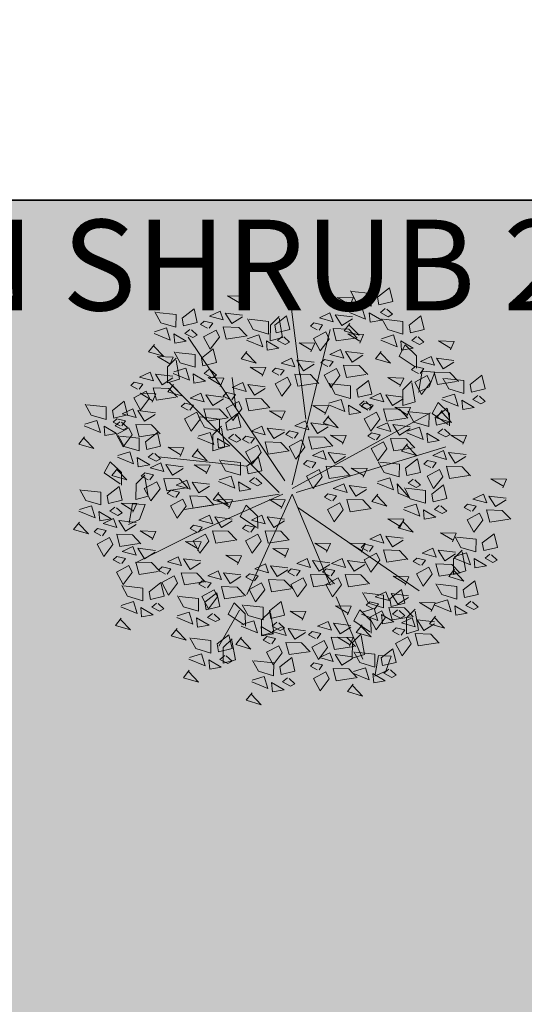
# Model space of a CAD drawing. Units: inches. Extents: x 1704 to 6393, y -157 to 1172.
# Tile 73 of 122: x 1954 to 1987, y 980 to 1045. Entities that reach past the tile are written whole.
import ezdxf

# ---------------------------------------------------------------- set-up
doc = ezdxf.new("R2010")
doc.units = ezdxf.units.IN
doc.header["$MEASUREMENT"] = 0
for name, color, linetype, lineweight in [('A-ANNO-DIMS', 7, 'Continuous', 13), ('C-PROP', 7, 'Continuous', 35), ('L-shrub', 74, 'Continuous', 18)]:
    doc.layers.add(name, color=color, linetype=linetype, lineweight=lineweight)
doc.layers.add('L-HRDS-PATT', color=9, linetype='Continuous', lineweight=13, true_color=0xc5c1ba)
doc.styles.get("Standard").update_dxf_attribs({"font": 'arial.ttf'})
doc.dimstyles.get("Standard").update_dxf_attribs({"dimtxt": 6, "dimasz": 2, "dimexe": 0.18, "dimexo": 0.0625, "dimgap": 0.09, "dimtad": 0, "dimtih": 1, "dimtoh": 1, "dimdec": 1, "dimzin": 0, "dimdsep": 46, "dimlunit": 3, "dimtxsty": 'Standard', "dimblk": 'ARCHTICK', "dimcen": 0.09, "dimadec": 0, "dimazin": 0, "dimtfac": 1, "dimtdec": 1, "dimtofl": 0, "dimtmove": 0, "dimatfit": 3, "dimfxl": 1, "dimtolj": 1, "dimtzin": 0, "dimarcsym": 0})

# ---------------------------------------------------------------- blocks, each defined once
blk = doc.blocks.new('flower shrub 3')
at = {"layer": 'L-shrub'}
for p, q in [((-123.5, 236), (-109, 242.8)), ((-130.4, 216.9), (-123.5, 236)), ((-109.8, 240.6), (-114, 215.7)), ((-114, 215.7), (-130.4, 216.9)), ((-96, 214.8), (-80.2, 219.2)), ((-80.2, 219.2), (-80.3, 198.9)), ((71.1, 221.6), (86.9, 226)), ((75.6, 196.7), (71.1, 221.6)), ((86.9, 226), (86.9, 205.7)), ((-91.6, 189.9), (-96, 214.8)), ((86.9, 205.7), (75.5, 194.4)), ((-80.3, 198.9), (-91.6, 187.7)), ((-166.1, 183.2), (-150.2, 187.7)), ((-161.6, 158.3), (-166.1, 183.2)), ((-150.2, 187.7), (-150.3, 167.3)), ((-104.3, 171), (-104.5, 187)), ((-102.9, 185.4), (-82, 171.2)), ((21.4, 185.5), (37.3, 189.9)), ((25.9, 160.6), (21.4, 185.5)), ((37.3, 189.9), (37.2, 169.6)), ((-150.3, 167.3), (-161.6, 156.1)), ((-89.8, 156.8), (-104.3, 171)), ((-82, 171.2), (-89.8, 156.8)), ((37.2, 169.6), (25.8, 158.3)), ((58.3, 162), (58.1, 177.9)), ((59.8, 176.3), (80.7, 162.2)), ((72.8, 147.7), (58.3, 162)), ((80.7, 162.2), (72.8, 147.7)), ((-227, 106.5), (-211.2, 110.9)), ((-222.6, 81.6), (-227, 106.5)), ((-211.2, 110.9), (-211.3, 90.6)), ((-211.3, 90.6), (-222.6, 79.4)), ((42.5, 35.6), (42.3, 51.6)), ((43.9, 50), (64.8, 35.8)), ((188.1, 20.6), (195.1, 39.7)), ((195.1, 39.7), (209.5, 46.5)), ((208.7, 44.3), (204.5, 19.5)), ((57, 21.4), (42.5, 35.6)), ((64.8, 35.8), (57, 21.4)), ((184.1, 9.5), (199.9, 13.9)), ((204.5, 19.5), (188.1, 20.6)), ((199.9, 13.9), (199.8, -6.4)), ((188.5, -15.4), (184.1, 9.5)), ((199.8, -6.4), (188.5, -17.7)), ((218.7, -20.8), (218.5, -4.8)), ((220.1, -6.4), (241, -20.6)), ((233.2, -35), (218.7, -20.8)), ((241, -20.6), (233.2, -35)), ((84.7, -53.7), (100.5, -49.2)), ((100.5, -49.2), (100.4, -69.6)), ((89.1, -78.6), (84.7, -53.7)), ((100.4, -69.6), (89.1, -80.8)), ((-206, -97.5), (-206.1, -81.5)), ((-204.5, -83.1), (-183.6, -97.3)), ((-191.5, -111.7), (-206, -97.5)), ((-183.6, -97.3), (-191.5, -111.7)), ((-161.5, -112.4), (-145.7, -107.9)), ((-157.1, -137.2), (-161.5, -112.4)), ((-145.7, -107.9), (-145.8, -128.2)), ((-179.9, -131.8), (-165.5, -125)), ((-166.2, -127.1), (-170.5, -152)), ((-186.9, -150.9), (-179.9, -131.8)), ((-145.8, -128.2), (-157.1, -139.5)), ((143.4, -141.7), (159.2, -137.2)), ((159.2, -137.2), (159.2, -157.6)), ((-170.5, -152), (-186.9, -150.9)), ((147.8, -166.6), (143.4, -141.7)), ((-163.1, -171.9), (-163.2, -156)), ((-161.6, -157.6), (-140.7, -171.7)), ((159.2, -157.6), (147.8, -168.8)), ((-148.6, -186.2), (-163.1, -171.9)), ((-140.7, -171.7), (-148.6, -186.2)), ((10.1, -195.8), (26, -191.4)), ((14.6, -220.7), (10.1, -195.8)), ((26, -191.4), (25.9, -211.7)), ((25.9, -211.7), (14.5, -223))]:
    blk.add_line(p, q, dxfattribs=at)
for points in [[(-81.5, 253.1), (-74, 262.7), (-93.5, 268.4), (-80.9, 255.3)], [(49.5, 264.4), (57, 273.9), (37.6, 279.7), (50.2, 266.6)], [(-50.4, 246.2), (-38.7, 261.6), (-30.1, 245.6), (-46.1, 237), (-50.4, 246.2)], [(3.7, 245), (10, 250.2), (-0.2, 255.6), (-5.8, 252.5), (1.6, 245.7)], [(24.3, 250.7), (23.1, 262.8), (8.2, 260.2), (24.3, 250.7)], [(49.4, 248), (33.8, 243.2), (29, 258.7), (50, 250.1)], [(-127.3, 233.7), (-121, 238.9), (-131.2, 244.3), (-136.8, 241.3), (-129.5, 234.4)], [(-106.8, 239.4), (-107.9, 251.5), (-122.8, 248.9), (-106.8, 239.4)], [(-81.7, 236.7), (-97.2, 231.9), (-102, 247.4), (-81, 238.9)], [(-84.3, 244.8), (-59.4, 248.7), (-55.3, 232.7), (-75.6, 233.3), (-86.6, 244.9)], [(130.8, 235.1), (138.4, 244.6), (118.9, 250.4), (131.5, 237.2)], [(-84.4, 211.6), (-109.5, 214.3), (-109.3, 230.8), (-89.8, 225), (-82.2, 211)], [(-37.1, 234.5), (-41.8, 227.9), (-30.6, 225.3), (-26, 229.7), (-34.9, 234.5)], [(13.5, 230.4), (-1.8, 218.4), (-6, 236.1), (11.8, 240.3), (13.5, 230.4)], [(46.7, 222.9), (21.5, 225.6), (21.7, 242.1), (41.2, 236.3), (48.8, 222.3)], [(105.6, 221.4), (104.4, 233.5), (89.5, 230.8), (105.6, 221.4)], [(-117.5, 219.1), (-132.8, 207.1), (-137, 224.8), (-119.3, 229), (-117.5, 219.1)], [(-59.4, 140), (-93.7, 220.8)], [(-80.5, 219.9), (-66.7, 228.5), (-58, 214.8), (-80.5, 217.6)], [(-55.5, 223.7), (-51.3, 212.3), (-37.6, 218.7), (-55.5, 223.7)], [(-48.1, 205.5), (-36.4, 221), (-27.8, 205), (-43.9, 196.4), (-48.1, 205.5)], [(10.6, 212.3), (22.3, 227.8), (30.9, 211.8), (14.9, 203.2), (10.6, 212.3)], [(85, 215.7), (91.3, 220.9), (81.1, 226.3), (75.5, 223.2), (82.9, 216.3)], [(130.7, 218.7), (115.1, 213.8), (110.3, 229.4), (131.3, 220.8)], [(-156.6, 201), (-144.8, 216.5), (-136.2, 200.5), (-152.3, 191.9), (-156.6, 201)], [(-82.1, 204.2), (-57.1, 208), (-53, 192.1), (-73.3, 192.7), (-84.3, 204.3)], [(-76.4, 204), (-81.2, 192.8), (-60.9, 192.3), (-76.4, 201.7)], [(-23.3, 211), (1.6, 214.8), (5.7, 198.9), (-14.6, 199.5), (-25.6, 211)], [(63.1, 192.2), (70.6, 201.7), (51.1, 207.5), (63.7, 194.4)], [(94.8, 201), (79.5, 189.1), (75.4, 206.8), (93.1, 211), (94.8, 201)], [(128, 193.6), (102.9, 196.3), (103, 212.7), (122.5, 207), (130.1, 192.9)], [(-190.5, 199.7), (-165.5, 203.5), (-161.4, 187.6), (-181.8, 188.2), (-192.7, 199.8)], [(-92.8, 176.4), (-85.3, 186), (-104.8, 191.7), (-92.2, 178.6)], [(-34.9, 193.9), (-39.6, 187.3), (-28.3, 184.7), (-23.7, 189.1), (-32.6, 193.8)], [(-19.5, 186), (-5.7, 194.7), (3, 180.9), (-19.5, 183.8)], [(23.9, 200.7), (19.2, 194), (30.4, 191.5), (35, 195.9), (26.1, 200.6)], [(65.7, 157.2), (92.6, 203.7)], [(146.6, 180.9), (154.2, 190.5), (134.7, 196.2), (147.3, 183.1)], [(-187.7, 165.1), (-180.1, 174.7), (-199.6, 180.4), (-187, 167.3)], [(-186.6, 174.8), (-172.8, 183.4), (-164.2, 169.6), (-186.7, 172.5)], [(-161.7, 178.6), (-157.5, 167.2), (-143.7, 173.6), (-161.7, 178.6)], [(-143.3, 189.4), (-148, 182.7), (-136.8, 180.2), (-132.1, 184.6), (-141, 189.3)], [(-122.7, 167.2), (-111, 182.7), (-102.3, 166.6), (-118.4, 158), (-122.7, 167.2)], [(-78.2, 179.3), (-64.4, 187.9), (-55.7, 174.2), (-78.3, 177)], [(-53.2, 183.1), (-49, 171.7), (-35.3, 178.1), (-53.2, 183.1)], [(5.5, 189.9), (9.7, 178.5), (23.4, 184.9), (5.5, 189.9)], [(17.3, 172.8), (23.5, 178), (13.3, 183.4), (7.7, 180.4), (15.1, 173.5)], [(37.8, 178.5), (36.7, 190.6), (21.8, 188), (37.8, 178.5)], [(62.9, 175.8), (47.4, 171), (42.5, 186.5), (63.6, 177.9)], [(121.4, 167.2), (120.3, 179.3), (105.3, 176.7), (121.4, 167.2)], [(218.9, 167.4), (226.5, 176.9), (207, 182.7), (219.6, 169.6)], [(-156.6, 165.8), (-131.6, 169.7), (-127.5, 153.8), (-147.9, 154.3), (-158.9, 165.9)], [(-138.6, 157), (-132.3, 162.2), (-142.5, 167.6), (-148.1, 164.6), (-140.8, 157.7)], [(-118.1, 162.7), (-119.2, 174.8), (-134.1, 172.2), (-118.1, 162.7)], [(-92.9, 160), (-108.5, 155.2), (-113.3, 170.7), (-92.3, 162.2)], [(-15.4, 170.1), (-20.2, 159), (0.1, 158.4), (-15.4, 167.9)], [(27.1, 158.2), (11.8, 146.2), (7.6, 163.9), (25.3, 168.1), (27.1, 158.2)], [(60.2, 150.7), (35.1, 153.4), (35.3, 169.9), (54.7, 164.1), (62.4, 150.1)], [(100.9, 161.5), (107.1, 166.7), (96.9, 172.1), (91.3, 169.1), (98.7, 162.2)], [(146.5, 164.5), (130.9, 159.7), (126.1, 175.2), (147.1, 166.7)], [(193.7, 153.7), (192.5, 165.8), (177.6, 163.1), (193.7, 153.7)], [(-233.5, 145.7), (-227.2, 151), (-237.4, 156.3), (-243, 153.3), (-235.6, 146.4)], [(-212.9, 151.4), (-214.1, 163.5), (-229, 160.9), (-212.9, 151.4)], [(-187.8, 148.7), (-203.4, 143.9), (-208.2, 159.4), (-187.2, 150.9)], [(-182.5, 158.9), (-187.4, 147.7), (-167, 147.1), (-182.6, 156.6)], [(-95.7, 134.9), (-120.8, 137.6), (-120.6, 154.1), (-101.1, 148.3), (-93.5, 134.3)], [(-109.4, 155.5), (-114.1, 148.9), (-102.9, 146.3), (-98.3, 150.7), (-107.2, 155.5)], [(-74.1, 163.4), (-78.9, 152.2), (-58.6, 151.7), (-74.2, 161.1)], [(110.7, 146.9), (95.3, 134.9), (91.2, 152.6), (108.9, 156.8), (110.7, 146.9)], [(94.2, 140.1), (105.9, 155.6), (114.5, 139.6), (98.5, 131), (94.2, 140.1)], [(143.8, 139.4), (118.7, 142.1), (118.8, 158.6), (138.3, 152.8), (146, 138.8)], [(173.1, 148), (179.4, 153.2), (169.2, 158.6), (163.6, 155.5), (171, 148.6)], [(218.8, 151), (203.2, 146.2), (198.4, 161.7), (219.4, 153.1)], [(-223.7, 131.1), (-239, 119.1), (-243.2, 136.9), (-225.4, 141), (-223.7, 131.1)], [(-190.5, 123.6), (-215.6, 126.4), (-215.5, 142.8), (-196, 137), (-188.4, 123)], [(-152.8, 140.9), (-139, 149.6), (-130.3, 135.8), (-152.8, 138.7)], [(-128.8, 142.4), (-144.1, 130.4), (-148.3, 148.1), (-130.6, 152.3), (-128.8, 142.4)], [(-127.8, 144.8), (-123.6, 133.4), (-109.9, 139.8), (-127.8, 144.8)], [(33.2, 131.1), (44.9, 146.6), (53.5, 130.5), (37.5, 121.9), (33.2, 131.1)], [(60.3, 138.8), (85.2, 142.6), (89.3, 126.7), (69, 127.3), (58, 138.8)], [(182.9, 133.3), (167.6, 121.4), (163.4, 139.1), (181.2, 143.3), (182.9, 133.3)], [(216.1, 125.9), (191, 128.6), (191.1, 145), (210.6, 139.3), (218.2, 125.2)], [(-9.9, 24.3), (-166.8, 132)], [(-66.2, 124.3), (-54.5, 139.8), (-45.9, 123.8), (-61.9, 115.2), (-66.2, 124.3)], [(-21, 124.3), (-9.3, 139.8), (-0.7, 123.8), (-16.7, 115.2), (-21, 124.3)], [(-0.7, 129.8), (24.2, 133.6), (28.3, 117.7), (8, 118.2), (-3, 129.8)], [(-2.5, 7.1), (56.3, 136.9)], [(107.4, 128.5), (102.7, 121.8), (114, 119.3), (118.6, 123.7), (109.7, 128.4)], [(146.1, 122.1), (157.9, 137.6), (166.5, 121.5), (150.4, 112.9), (146.1, 122.1)], [(-212.5, 104.2), (-205, 113.8), (-224.5, 119.5), (-211.9, 106.4)], [(-183.7, 110.8), (-171.9, 126.3), (-163.3, 110.2), (-179.4, 101.6), (-183.7, 110.8)], [(-148.7, 125), (-153.5, 113.9), (-133.2, 113.3), (-148.7, 122.8)], [(-100.1, 123), (-75.2, 126.8), (-71.1, 110.9), (-91.4, 111.5), (-102.4, 123)], [(-54.9, 123), (-30, 126.8), (-25.9, 110.9), (-46.2, 111.5), (-57.2, 123)], [(-2.5, 7.1), (-51.6, 124.7)], [(46.4, 119.4), (41.7, 112.8), (53, 110.2), (57.6, 114.6), (48.7, 119.4)], [(64.1, 113.8), (77.9, 122.5), (86.6, 108.7), (64, 111.6)], [(89.1, 117.7), (93.3, 106.3), (107, 112.7), (89.1, 117.7)], [(112.2, 120.7), (137.2, 124.6), (141.3, 108.7), (120.9, 109.2), (110, 120.8)], [(204.9, 108.5), (216.6, 124), (225.2, 108), (209.2, 99.4), (204.9, 108.5)], [(-237.8, 90.5), (-238.9, 102.6), (-253.8, 100), (-237.8, 90.5)], [(-217.6, 109.4), (-192.6, 113.3), (-188.5, 97.4), (-208.9, 97.9), (-219.9, 109.5)], [(-115.9, 92.7), (-104.2, 108.2), (-95.6, 92.2), (-111.6, 83.6), (-115.9, 92.7)], [(-96.3, 98.1), (-82.5, 106.7), (-73.8, 92.9), (-96.3, 95.8)], [(-53, 112.7), (-57.6, 106), (-46.4, 103.5), (-41.8, 107.9), (-50.7, 112.6)], [(-51.1, 98.1), (-37.3, 106.7), (-28.6, 92.9), (-51.2, 95.8)], [(-7.8, 112.7), (-12.5, 106), (-1.2, 103.5), (3.4, 107.9), (-5.5, 112.6)], [(3.1, 104.8), (16.9, 113.5), (25.6, 99.7), (3.1, 102.6)], [(28.1, 108.7), (32.3, 97.3), (46, 103.7), (28.1, 108.7)], [(116.1, 95.8), (129.9, 104.5), (138.5, 90.7), (116, 93.5)], [(159.4, 110.4), (154.7, 103.8), (165.9, 101.2), (170.6, 105.6), (161.6, 110.4)], [(170.9, 107.2), (195.9, 111), (200, 95.1), (179.7, 95.7), (168.7, 107.3)], [(-258.3, 84.8), (-252.1, 90), (-262.2, 95.4), (-267.9, 92.4), (-260.5, 85.5)], [(-212.7, 87.8), (-228.2, 83), (-233.1, 98.5), (-212, 90)], [(-213.7, 84.5), (-200, 93.2), (-191.3, 79.4), (-213.8, 82.3)], [(-170.4, 99.1), (-175.1, 92.5), (-163.9, 89.9), (-159.2, 94.3), (-168.2, 99.1)], [(-149.8, 91.4), (-124.9, 95.2), (-120.8, 79.3), (-141.1, 79.9), (-152.1, 91.5)], [(-71.3, 101.9), (-67.1, 90.5), (-53.4, 96.9), (-71.3, 101.9)], [(-26.1, 101.9), (-21.9, 90.5), (-8.2, 96.9), (-26.1, 101.9)], [(68.2, 97.9), (63.4, 86.8), (83.7, 86.2), (68.1, 95.7)], [(122.1, 56.8), (200.5, 95.9)], [(141, 99.6), (145.2, 88.2), (159, 94.6), (141, 99.6)], [(174.8, 82.3), (188.6, 90.9), (197.3, 77.1), (174.7, 80)], [(218.1, 96.9), (213.4, 90.2), (224.7, 87.7), (229.3, 92.1), (220.4, 96.8)], [(-248.5, 70.2), (-263.8, 58.2), (-268, 75.9), (-250.3, 80.1), (-248.5, 70.2)], [(-215.4, 62.7), (-240.5, 65.4), (-240.3, 81.9), (-220.8, 76.1), (-213.2, 62.1)], [(-188.8, 88.4), (-184.6, 77), (-170.8, 83.4), (-188.8, 88.4)], [(-102.6, 81.1), (-107.3, 74.5), (-96.1, 71.9), (-91.5, 76.3), (-100.4, 81)], [(-92.2, 82.1), (-97, 71), (-76.7, 70.4), (-92.3, 79.9)], [(-47, 82.1), (-51.8, 71), (-31.5, 70.4), (-47.1, 79.9)], [(7.2, 88.9), (2.4, 77.8), (22.7, 77.2), (7.1, 86.7)], [(37.7, 67.9), (49.4, 83.4), (58, 67.4), (42, 58.8), (37.7, 67.9)], [(105.5, 67.9), (117.2, 83.4), (125.8, 67.4), (109.8, 58.8), (105.5, 67.9)], [(120.2, 79.9), (115.3, 68.7), (135.7, 68.2), (120.1, 77.6)], [(199.8, 86.1), (204, 74.7), (217.7, 81.1), (199.8, 86.1)], [(229.7, 72.4), (241.4, 87.9), (250.1, 71.9), (234, 63.3), (229.7, 72.4)], [(-209.7, 68.6), (-214.5, 57.5), (-194.2, 56.9), (-209.7, 66.3)], [(-146, 66.5), (-132.2, 75.1), (-123.5, 61.3), (-146, 64.2)], [(-121, 70.3), (-116.8, 58.9), (-103.1, 65.3), (-121, 70.3)], [(3.8, 66.6), (28.7, 70.4), (32.8, 54.5), (12.5, 55.1), (1.5, 66.6)], [(71.6, 66.6), (96.5, 70.4), (100.6, 54.5), (80.3, 55.1), (69.3, 66.6)], [(178.9, 66.3), (174.1, 55.2), (194.4, 54.6), (178.8, 64.1)], [(195.8, 71.1), (220.8, 74.9), (224.8, 59), (204.5, 59.6), (193.5, 71.2)], [(-249.2, 40.8), (-237.5, 56.3), (-228.8, 40.3), (-244.9, 31.7), (-249.2, 40.8)], [(-147, 41), (-139.5, 50.6), (-159, 56.4), (-146.4, 43.2)], [(9.7, 7.1), (125, 58.6)], [(51, 56.3), (46.3, 49.6), (57.5, 47.1), (62.1, 51.5), (53.2, 56.2)], [(118.7, 56.3), (114, 49.6), (125.3, 47.1), (129.9, 51.5), (121, 56.2)], [(199.6, 46.2), (213.4, 54.8), (222.1, 41), (199.6, 43.9)], [(243, 60.8), (238.3, 54.1), (249.5, 51.6), (254.1, 56), (245.2, 60.7)], [(273.1, 43.3), (280.7, 52.8), (261.2, 58.6), (273.8, 45.5)], [(-283.1, 39.5), (-258.1, 43.3), (-254.1, 27.4), (-274.4, 28), (-285.4, 39.6)], [(-172.3, 27.3), (-173.4, 39.4), (-188.3, 36.8), (-172.3, 27.3)], [(-141.9, 50.6), (-146.7, 39.4), (-126.4, 38.9), (-141.9, 48.3)], [(-68.5, 27.3), (-56.7, 42.8), (-48.1, 26.8), (-64.2, 18.2), (-68.5, 27.3)], [(7.6, 41.6), (21.4, 50.3), (30.1, 36.5), (7.6, 39.4)], [(32.6, 45.5), (36.8, 34.1), (50.5, 40.5), (32.6, 45.5)], [(75.4, 41.6), (89.2, 50.3), (97.9, 36.5), (75.3, 39.4)], [(100.4, 45.5), (104.6, 34.1), (118.3, 40.5), (100.4, 45.5)], [(134.9, 22.8), (146.6, 38.3), (155.2, 22.2), (139.1, 13.7), (134.9, 22.8)], [(224.6, 50), (228.8, 38.6), (242.5, 45), (224.6, 50)], [(247.9, 29.6), (246.8, 41.7), (231.8, 39.1), (247.9, 29.6)], [(-235.9, 29.2), (-240.6, 22.6), (-229.4, 20), (-224.8, 24.4), (-233.7, 29.1)], [(-192.8, 21.7), (-186.5, 26.9), (-196.7, 32.2), (-202.4, 29.2), (-195, 22.3)], [(-147.2, 24.6), (-162.7, 19.8), (-167.5, 35.4), (-146.5, 26.8)], [(-102.4, 26), (-77.4, 29.8), (-73.3, 13.9), (-93.7, 14.4), (-104.6, 26)], [(11.7, 25.7), (6.9, 14.6), (27.2, 14), (11.7, 23.5)], [(14.6, 7.1), (137.2, 26.7)], [(79.5, 25.7), (74.7, 14.6), (95, 14), (79.4, 23.5)], [(203.7, 30.3), (198.9, 19.1), (219.2, 18.5), (203.7, 28)], [(227.4, 23.9), (233.6, 29.1), (223.4, 34.5), (217.8, 31.4), (225.2, 24.6)], [(273, 26.9), (257.4, 22.1), (252.6, 37.6), (273.6, 29)], [(-279.3, 14.6), (-265.5, 23.2), (-256.8, 9.5), (-279.3, 12.3)], [(-254.3, 18.4), (-250.1, 7), (-236.4, 13.4), (-254.3, 18.4)], [(-183, 7), (-198.3, -4.9), (-202.5, 12.8), (-184.8, 16.9), (-183, 7)], [(-149.9, -0.5), (-175, 2.3), (-174.8, 18.7), (-155.3, 12.9), (-147.7, -1.1)], [(-113.1, 7.2), (-105.6, 16.7), (-125.1, 22.5), (-112.5, 9.4)], [(-55.2, 15.7), (-59.9, 9), (-48.7, 6.5), (-44, 10.9), (-53, 15.6)], [(92.4, 4.9), (100, 14.5), (80.5, 20.3), (93.1, 7.1)], [(100.9, 21.5), (125.9, 25.3), (130, 9.4), (109.6, 9.9), (98.7, 21.5)], [(168.7, 0.2), (180.5, 15.7), (189.1, -0.3), (173, -8.9), (168.7, 0.2)], [(237.2, 9.2), (221.8, -2.7), (217.7, 15), (235.4, 19.2), (237.2, 9.2)], [(270.3, 1.8), (245.2, 4.5), (245.3, 20.9), (264.8, 15.2), (272.5, 1.2)], [(-7.4, 4.7), (-201.1, -54.1)], [(-138.4, -6.5), (-139.5, 5.6), (-154.3, 11.9), (-138.4, -6.5)], [(-113.3, -9.2), (-128.8, -14), (-133.7, 1.5), (-112.6, -7.1)], [(-98.5, 1), (-84.7, 9.7), (-76.1, -4.1), (-98.6, -1.2)], [(-73.6, 4.9), (-69.4, -6.5), (-55.6, -0.1), (-73.6, 4.9)], [(14.6, 4.7), (156.8, -137.4)], [(67.2, -8.8), (66, 3.3), (51.1, 0.7), (67.2, -8.8)], [(104.8, -3.5), (118.6, 5.2), (127.2, -8.6), (104.7, -5.7)], [(129.7, 0.4), (133.9, -11), (147.7, -4.6), (129.7, 0.4)], [(134.8, -1.1), (159.8, 2.7), (163.9, -13.2), (143.5, -12.6), (132.5, -1)], [(148.1, 11.2), (143.4, 4.5), (154.6, 2), (159.3, 6.3), (150.4, 11.1)], [(-275.2, -1.3), (-280, -12.5), (-259.7, -13), (-275.2, -3.6)], [(-197.2, -15.6), (-185.5, -0.1), (-176.9, -16.1), (-192.9, -24.7), (-197.2, -15.6)], [(-2.5, -0.2), (-181.5, -98.2)], [(-158.9, -12.2), (-152.7, -7), (-162.9, -1.6), (-168.5, -4.7), (-161.1, -11.5)], [(-2.5, -5.1), (-51.6, -205.9)], [(-41.3, -15.6), (-29.6, -0.1), (-21, -16.1), (-37.1, -24.7), (-41.3, -15.6)], [(7.3, -10), (132.3, -196.1)], [(46.6, -14.4), (52.9, -9.2), (42.7, -3.9), (37.1, -6.9), (44.5, -13.8)], [(92.3, -11.5), (76.7, -16.3), (71.9, -0.7), (92.9, -9.3)], [(182, -11.4), (177.3, -18.1), (188.5, -20.6), (193.1, -16.2), (184.2, -11.5)], [(223.5, -26.6), (231, -17.1), (211.5, -11.3), (224.1, -24.5)], [(-231.1, -16.9), (-206.2, -13.1), (-202.1, -29), (-222.4, -28.4), (-233.4, -16.8)], [(-149.1, -26.8), (-164.4, -38.8), (-168.6, -21.1), (-150.9, -16.9), (-149.1, -26.8)], [(-116, -34.3), (-141.1, -31.6), (-140.9, -15.2), (-121.5, -20.9), (-113.8, -34.9)], [(-94.4, -14.9), (-99.3, -26), (-78.9, -26.6), (-94.5, -17.1)], [(-75.3, -16.9), (-50.3, -13.1), (-46.2, -29), (-66.6, -28.4), (-77.5, -16.8)], [(56.4, -29.1), (41.1, -41), (36.9, -23.3), (54.7, -19.2), (56.4, -29.1)], [(89.6, -36.6), (64.5, -33.8), (64.6, -17.4), (84.1, -23.2), (91.7, -37.2)], [(108.9, -19.4), (104, -30.5), (124.4, -31.1), (108.8, -21.6)], [(138.6, -26), (152.4, -17.4), (161.1, -31.2), (138.6, -28.3)], [(163.6, -22.2), (167.8, -33.6), (181.6, -27.2), (163.6, -22.2)], [(-227.3, -41.8), (-213.5, -33.2), (-204.8, -46.9), (-227.4, -44.1)], [(-202.3, -38), (-198.1, -49.4), (-184.4, -43), (-202.3, -38)], [(-184, -27.2), (-188.7, -33.8), (-177.4, -36.4), (-172.8, -32), (-181.7, -27.3)], [(-124.9, -51.7), (-113.2, -36.2), (-104.6, -52.2), (-120.7, -60.8), (-124.9, -51.7)], [(-71.4, -41.8), (-57.6, -33.2), (-49, -46.9), (-71.5, -44.1)], [(-46.5, -38), (-42.3, -49.4), (-28.5, -43), (-46.5, -38)], [(-28.1, -27.2), (-32.8, -33.8), (-21.6, -36.4), (-16.9, -32), (-25.8, -27.3)], [(37.7, -47.1), (49.4, -31.7), (58, -47.7), (42, -56.3), (37.7, -47.1)], [(55.9, -29), (171.1, -41.2)], [(119.5, -51.5), (127.1, -41.9), (107.6, -36.2), (120.2, -49.3)], [(177.7, -46), (183.9, -40.8), (173.7, -35.5), (168.1, -38.5), (175.5, -45.4)], [(198.2, -40.3), (197.1, -28.2), (182.1, -30.9), (198.2, -40.3)], [(223.3, -43.1), (207.7, -47.9), (202.9, -32.3), (223.9, -40.9)], [(-151.5, -58.2), (-144, -48.7), (-163.5, -42.9), (-150.9, -56.1)], [(-158.9, -53), (-133.9, -49.2), (-129.8, -65.1), (-150.1, -64.5), (-161.1, -52.9)], [(-18.8, -53.9), (-7, -38.4), (1.6, -54.5), (-14.5, -63.1), (-18.8, -53.9)], [(3.8, -48.5), (28.7, -44.6), (32.8, -60.6), (12.5, -60), (1.5, -48.4)], [(142.7, -41.9), (137.9, -53.1), (158.2, -53.6), (142.7, -44.2)], [(187.5, -60.7), (172.1, -72.6), (168, -54.9), (185.7, -50.8), (187.5, -60.7)], [(220.6, -68.1), (195.5, -65.4), (195.6, -49), (215.1, -54.8), (222.8, -68.8)], [(-223.2, -57.7), (-228, -68.9), (-207.7, -69.4), (-223.3, -60)], [(-176.8, -71.9), (-177.9, -59.8), (-192.8, -62.5), (-176.8, -71.9)], [(-111.7, -63.3), (-116.4, -69.9), (-105.2, -72.5), (-100.5, -68.1), (-109.4, -63.4)], [(-67.3, -57.7), (-72.2, -68.9), (-51.8, -69.4), (-67.4, -60)], [(-52.7, -55.3), (-27.7, -51.4), (-23.6, -67.3), (-44, -66.8), (-54.9, -55.2)], [(51, -58.8), (46.3, -65.4), (57.5, -68), (62.1, -63.6), (53.2, -58.8)], [(73.8, -70.8), (80, -65.6), (69.8, -60.3), (64.2, -63.3), (71.6, -70.2)], [(94.3, -65.2), (93.2, -53.1), (78.2, -55.7), (94.3, -65.2)], [(119.4, -67.9), (103.8, -72.7), (99, -57.1), (120, -65.7)], [(204.9, -69.7), (216.6, -54.2), (225.2, -70.3), (209.2, -78.8), (204.9, -69.7)], [(266.4, -67.2), (273.9, -57.7), (254.4, -51.9), (267, -65.1)], [(-197.3, -77.6), (-191.1, -72.4), (-201.3, -67), (-206.9, -70.1), (-199.5, -77)], [(-151.7, -74.6), (-167.2, -79.5), (-172.1, -63.9), (-151, -72.5)], [(-155, -77.9), (-141.2, -69.3), (-132.6, -83), (-155.1, -80.2)], [(-130.1, -74.1), (-125.8, -85.5), (-112.1, -79.1), (-130.1, -74.1)], [(-115.9, -90), (-104.2, -74.5), (-95.6, -90.6), (-111.6, -99.2), (-115.9, -90)], [(-48.8, -80.2), (-35.1, -71.5), (-26.4, -85.3), (-48.9, -82.4)], [(-23.9, -76.3), (-19.7, -87.7), (-5.9, -81.3), (-23.9, -76.3)], [(-5.5, -65.6), (-10.2, -72.2), (1, -74.8), (5.7, -70.4), (-3.3, -65.6)], [(7.6, -73.4), (21.4, -64.8), (30.1, -78.5), (7.6, -75.7)], [(32.6, -69.6), (36.8, -81), (50.5, -74.6), (32.6, -69.6)], [(83.6, -85.5), (68.2, -97.4), (64.1, -79.7), (81.8, -75.6), (83.6, -85.5)], [(116.7, -93), (91.6, -90.2), (91.7, -73.8), (111.2, -79.6), (118.8, -93.6)], [(116.8, -90), (128.5, -74.5), (137.1, -90.6), (121.1, -99.2), (116.8, -90)], [(170.9, -71), (195.9, -67.2), (200, -83.1), (179.7, -82.6), (168.7, -71)], [(220.6, -86.6), (226.8, -81.4), (216.6, -76.1), (211, -79.1), (218.4, -86)], [(241.1, -80.9), (240, -68.9), (225.1, -71.5), (241.1, -80.9)], [(266.2, -83.7), (250.7, -88.5), (245.8, -72.9), (266.9, -81.5)], [(-196.7, -101.1), (-189.2, -91.6), (-208.7, -85.8), (-196.1, -98.9)], [(-187.5, -92.3), (-202.8, -104.2), (-207, -86.5), (-189.3, -82.3), (-187.5, -92.3)], [(-154.4, -99.7), (-179.5, -97), (-179.3, -80.6), (-159.9, -86.3), (-152.2, -100.4)], [(-149.8, -91.4), (-124.9, -87.5), (-120.8, -103.4), (-141.1, -102.9), (-152.1, -91.3)], [(-49.9, -94.3), (-42.3, -84.8), (-61.8, -79), (-49.2, -92.2)], [(62.6, -103.5), (74.3, -88.1), (82.9, -104.1), (66.8, -112.7), (62.6, -103.5)], [(82.8, -91.4), (107.8, -87.5), (111.9, -103.4), (91.6, -102.9), (80.6, -91.3)], [(174.8, -96), (188.6, -87.3), (197.3, -101.1), (174.7, -98.2)], [(218.1, -81.3), (213.4, -88), (224.7, -90.6), (229.3, -86.2), (220.4, -81.4)], [(-150.9, -93.8), (-155.7, -105), (-135.4, -105.5), (-151, -96.1)], [(-102.6, -101.7), (-107.3, -108.3), (-96.1, -110.9), (-91.5, -106.5), (-100.4, -101.7)], [(-75.1, -108), (-76.3, -95.9), (-91.2, -98.6), (-75.1, -108)], [(-50, -110.7), (-65.6, -115.6), (-70.4, -100), (-49.4, -108.6)], [(-44.8, -96.1), (-49.6, -107.2), (-29.3, -107.8), (-44.8, -98.3)], [(-12.8, -149), (-20.2, -90.2)], [(11.7, -89.3), (6.9, -100.5), (27.2, -101), (11.7, -91.6)], [(28.6, -104.9), (53.6, -101), (57.7, -117), (37.4, -116.4), (26.4, -104.8)], [(130, -101.7), (125.3, -108.3), (136.6, -110.9), (141.2, -106.5), (132.3, -101.7)], [(182.3, -117.1), (194, -101.6), (202.6, -117.6), (186.6, -126.2), (182.3, -117.1)], [(199.8, -92.1), (204, -103.5), (217.7, -97.1), (199.8, -92.1)], [(230.4, -101.3), (215.1, -113.2), (210.9, -95.5), (228.6, -91.4), (230.4, -101.3)], [(263.5, -108.8), (238.4, -106), (238.6, -89.6), (258, -95.4), (265.7, -109.4)], [(-242.5, -120.5), (-236.2, -115.3), (-246.4, -109.9), (-252, -112.9), (-244.7, -119.8)], [(-222, -114.8), (-223.1, -102.7), (-238, -105.3), (-222, -114.8)], [(-196.9, -117.5), (-212.4, -122.3), (-217.2, -106.8), (-196.2, -115.4)], [(-146, -116.3), (-132.2, -107.6), (-123.5, -121.4), (-146, -118.5)], [(-121, -112.4), (-116.8, -123.8), (-103.1, -117.4), (-121, -112.4)], [(-95.7, -113.7), (-89.4, -108.5), (-99.6, -103.1), (-105.2, -106.2), (-97.8, -113.1)], [(70.6, -104.9), (75.5, -144.1)], [(86.7, -116.3), (100.5, -107.6), (109.2, -121.4), (86.6, -118.5)], [(111.7, -112.4), (115.9, -123.8), (129.6, -117.4), (111.7, -112.4)], [(148.4, -118.4), (173.3, -114.6), (177.4, -130.5), (157.1, -129.9), (146.1, -118.4)], [(178.9, -111.9), (174.1, -123), (194.4, -123.6), (178.8, -114.1)], [(-232.7, -135.1), (-248, -147.1), (-252.2, -129.4), (-234.5, -125.2), (-232.7, -135.1)], [(-199.6, -142.6), (-224.7, -139.9), (-224.5, -123.4), (-205, -129.2), (-197.4, -143.2)], [(-181.4, -137.4), (-169.7, -121.9), (-161.1, -137.9), (-177.1, -146.5), (-181.4, -137.4)], [(-85.9, -128.4), (-101.2, -140.3), (-105.4, -122.6), (-87.6, -118.4), (-85.9, -128.4)], [(-52.7, -135.8), (-77.8, -133.1), (-77.7, -116.7), (-58.2, -122.4), (-50.6, -136.5)], [(-0.7, -135.1), (11, -119.7), (19.6, -135.7), (3.6, -144.3), (-0.7, -135.1)], [(32.5, -129.8), (46.3, -121.2), (54.9, -134.9), (32.4, -132.1)], [(57.4, -126), (61.7, -137.4), (75.4, -131), (57.4, -126)], [(75.8, -115.2), (71.1, -121.8), (82.3, -124.4), (87, -120), (78.1, -115.3)], [(151.2, -134.9), (158.7, -125.4), (139.2, -119.6), (151.8, -132.8)], [(-215.3, -138.7), (-190.4, -134.9), (-186.3, -150.8), (-206.6, -150.3), (-217.6, -138.7)], [(-141.9, -132.2), (-146.7, -143.3), (-126.4, -143.9), (-141.9, -134.4)], [(-63.9, -146.4), (-52.2, -130.9), (-43.6, -147), (-59.7, -155.6), (-63.9, -146.4)], [(-34.6, -136.5), (-9.7, -132.6), (-5.6, -148.5), (-25.9, -148), (-36.9, -136.4)], [(90.8, -132.2), (86, -143.3), (106.3, -143.9), (90.7, -134.4)], [(125.9, -148.6), (124.8, -136.5), (109.9, -139.2), (125.9, -148.6)], [(152.2, -143.4), (166, -134.7), (174.7, -148.5), (152.1, -145.6)], [(177.2, -139.5), (181.4, -150.9), (195.1, -144.5), (177.2, -139.5)], [(195.5, -128.7), (190.8, -135.4), (202.1, -137.9), (206.7, -133.5), (197.8, -128.8)], [(-168.2, -149), (-172.9, -155.7), (-161.6, -158.2), (-157, -153.8), (-165.9, -149.1)], [(-97.9, -147.8), (-72.9, -143.9), (-68.8, -159.8), (-89.1, -159.3), (-100.1, -147.7)], [(-30.8, -161.4), (-17, -152.7), (-8.3, -166.5), (-30.8, -163.7)], [(-12.3, -147.2), (-0.1, -242.7)], [(12.6, -146.8), (7.9, -153.4), (19.1, -156), (23.7, -151.6), (14.8, -146.8)], [(36.6, -145.7), (31.7, -156.9), (52.1, -157.4), (36.5, -148)], [(105.4, -154.3), (111.6, -149.1), (101.4, -143.7), (95.8, -146.8), (103.2, -153.7)], [(151, -151.4), (135.5, -156.2), (130.6, -140.6), (151.7, -149.2)], [(-211.5, -163.7), (-197.7, -155), (-189, -168.8), (-211.5, -165.9)], [(-186.5, -159.8), (-182.3, -171.2), (-168.6, -164.8), (-186.5, -159.8)], [(-117.6, -177.8), (-110.1, -168.3), (-129.6, -162.5), (-117, -175.6)], [(-94, -172.7), (-80.2, -164), (-71.6, -177.8), (-94.1, -174.9)], [(-50.7, -158.1), (-55.4, -164.7), (-44.2, -167.3), (-39.5, -162.9), (-48.4, -158.1)], [(-5.8, -157.6), (-1.6, -169), (12.1, -162.6), (-5.8, -157.6)], [(56.3, -177.8), (63.8, -168.3), (44.3, -162.5), (56.9, -175.6)], [(115.2, -169), (99.9, -180.9), (95.7, -163.2), (113.4, -159.1), (115.2, -169)], [(148.3, -176.4), (123.2, -173.7), (123.3, -157.3), (142.8, -163.1), (150.5, -177.1)], [(156.3, -159.3), (151.5, -170.4), (171.8, -171), (156.2, -161.5)], [(-69.1, -168.8), (-64.8, -180.2), (-51.1, -173.8), (-69.1, -168.8)], [(-50.4, -193.8), (-38.7, -178.3), (-30.1, -194.3), (-46.1, -202.9), (-50.4, -193.8)], [(-26.7, -177.3), (-31.5, -188.5), (-11.2, -189), (-26.7, -179.6)], [(176, -186.8), (183.5, -177.3), (164.1, -171.5), (176.7, -184.7)], [(-207.4, -179.6), (-212.2, -190.7), (-191.9, -191.3), (-207.5, -181.8)], [(-163.4, -197.2), (-157.2, -192), (-167.4, -186.6), (-173, -189.7), (-165.6, -196.5)], [(-142.9, -191.5), (-144, -179.4), (-159, -182), (-142.9, -191.5)], [(-117.8, -194.2), (-133.4, -199), (-138.2, -183.5), (-117.2, -192.1)], [(-89.9, -188.6), (-94.8, -199.8), (-74.4, -200.3), (-90, -190.9)], [(10.5, -197.2), (16.8, -192), (6.6, -186.6), (1, -189.7), (8.3, -196.5)], [(31, -191.5), (29.9, -179.4), (15, -182), (31, -191.5)], [(56.1, -194.2), (40.6, -199), (35.8, -183.5), (56.8, -192.1)], [(91.9, -196.1), (103.6, -180.6), (112.3, -196.6), (96.2, -205.2), (91.9, -196.1)], [(150.8, -200.5), (149.6, -188.4), (134.7, -191.1), (150.8, -200.5)], [(-153.6, -211.9), (-169, -223.8), (-173.1, -206.1), (-155.4, -201.9), (-153.6, -211.9)], [(-120.5, -219.3), (-145.6, -216.6), (-145.5, -200.2), (-126, -205.9), (-118.3, -219.9)], [(-77, -213.9), (-69.5, -204.4), (-88.9, -198.6), (-76.3, -211.7)], [(-84.3, -195.1), (-59.4, -191.3), (-55.3, -207.2), (-75.6, -206.7), (-86.6, -195.1)], [(20.3, -211.9), (5, -223.8), (0.8, -206.1), (18.5, -201.9), (20.3, -211.9)], [(53.4, -219.3), (28.3, -216.6), (28.5, -200.2), (48, -205.9), (55.6, -219.9)], [(58, -197.4), (83, -193.6), (87.1, -209.5), (66.7, -208.9), (55.7, -197.3)], [(130.2, -206.2), (136.5, -201), (126.3, -195.6), (120.7, -198.7), (128.1, -205.6)], [(175.9, -203.3), (160.3, -208.1), (155.5, -192.5), (176.5, -201.1)], [(-102.2, -227.6), (-103.4, -215.5), (-118.3, -218.1), (-102.2, -227.6)], [(-80.5, -220.1), (-66.7, -211.4), (-58, -225.2), (-80.5, -222.3)], [(-55.5, -216.2), (-51.3, -227.6), (-37.6, -221.2), (-55.5, -216.2)], [(-37.1, -205.4), (-41.8, -212.1), (-30.6, -214.6), (-26, -210.3), (-34.9, -205.5)], [(61.8, -222.3), (75.6, -213.7), (84.3, -227.4), (61.8, -224.6)], [(105.2, -207.7), (100.5, -214.3), (111.7, -216.9), (116.3, -212.5), (107.4, -207.8)], [(140, -220.9), (124.7, -232.8), (120.5, -215.1), (138.3, -210.9), (140, -220.9)], [(173.2, -228.3), (148, -225.6), (148.2, -209.2), (167.7, -214.9), (175.3, -229)], [(-122.8, -233.3), (-116.5, -228.1), (-126.7, -222.7), (-132.3, -225.8), (-124.9, -232.6)], [(-77.1, -230.3), (-92.7, -235.1), (-97.5, -219.6), (-76.5, -228.2)], [(86.8, -218.5), (91, -229.9), (104.7, -223.5), (86.8, -218.5)], [(-113, -248), (-128.3, -259.9), (-132.5, -242.2), (-114.7, -238), (-113, -248)], [(-79.8, -255.4), (-105, -252.7), (-104.8, -236.3), (-85.3, -242), (-77.7, -256)], [(-76.4, -236), (-81.2, -247.1), (-60.9, -247.7), (-76.4, -238.2)], [(65.9, -238.2), (61.1, -249.4), (81.4, -249.9), (65.9, -240.5)]]:
    blk.add_lwpolyline(points, dxfattribs=at)
blk = doc.blocks.new('_ArchTick')
at = {"color": 0, "linetype": 'ByBlock', "const_width": 0.15}
blk.add_lwpolyline([(-0.5, -0.5), (0.5, 0.5)], dxfattribs=at)
blk = doc.blocks.new('*D80')
at = {"layer": 'A-ANNO-DIMS', "color": 0, "lineweight": -2, "transparency": 16777216}
for p, q in [((2018.966, 1028.916), (2016.966, 1028.916)), ((2018.966, 1025.001), (2018.966, 1029.096)), ((2045.487, 1028.916), (2018.966, 1028.916)), ((2045.487, 1025.001), (2045.487, 1029.096))]:
    blk.add_line(p, q, dxfattribs=at)
at = {"layer": 'Defpoints', "color": 0, "lineweight": -3, "transparency": 16777216}
for p in [(2018.966, 1028.916), (2018.966, 1024.938), (2045.487, 1024.938)]:
    blk.add_point(p, dxfattribs=at)
at = {"layer": 'A-ANNO-DIMS', "color": 0, "lineweight": -2, "transparency": 16777216, "xscale": 2, "yscale": 2, "zscale": 2, "rotation": 180}
blk.add_blockref('_ArchTick', (2018.966, 1028.916), dxfattribs=at)
at = {"layer": 'A-ANNO-DIMS', "color": 0, "lineweight": -2, "transparency": 16777216, "xscale": 2, "yscale": 2, "zscale": 2}
blk.add_blockref('_ArchTick', (2045.487, 1028.916), dxfattribs=at)
at = {"layer": 'A-ANNO-DIMS', "color": 0, "transparency": 16777216, "insert": (1967.173, 1028.916), "char_height": 6, "attachment_point": 5}
blk.add_mtext('\\A1;AUTUMN SHRUB 27 TYP.', dxfattribs=at)
blk = doc.blocks.new('*D94')
at = {"layer": 'A-ANNO-DIMS', "color": 0, "lineweight": -2, "transparency": 16777216}
for p, q in [((1898.349, 895.275), (1898.349, 1105.287)), ((1898.349, 1105.107), (1979.39, 1105.107)), ((2073.349, 1105.107), (1992.307, 1105.107)), ((2073.349, 895.275), (2073.349, 1105.287))]:
    blk.add_line(p, q, dxfattribs=at)
at = {"layer": 'Defpoints', "color": 0, "lineweight": -3, "transparency": 16777216}
for p in [(2073.349, 1105.107), (1898.349, 895.213), (2073.349, 895.213)]:
    blk.add_point(p, dxfattribs=at)
at = {"layer": 'A-ANNO-DIMS', "color": 0, "lineweight": -2, "transparency": 16777216, "xscale": 2, "yscale": 2, "zscale": 2, "rotation": 180}
blk.add_blockref('_ArchTick', (1898.349, 1105.107), dxfattribs=at)
at = {"layer": 'A-ANNO-DIMS', "color": 0, "lineweight": -2, "transparency": 16777216, "xscale": 2, "yscale": 2, "zscale": 2}
blk.add_blockref('_ArchTick', (2073.349, 1105.107), dxfattribs=at)
at = {"layer": 'A-ANNO-DIMS', "color": 0, "transparency": 16777216, "insert": (1985.849, 1105.107), "char_height": 6, "attachment_point": 5}
blk.add_mtext('\\A1;175', dxfattribs=at)

msp = doc.modelspace()

# ---------------------------------------------------------------- hatches: boundary and pattern name
at = {"layer": 'L-HRDS-PATT', "transparency": 33554643}
h = msp.add_hatch(color=256, dxfattribs=at)
h.dxf.hatch_style = 1
h.paths.add_polyline_path([(2065.589, 1033.213), (1898.349, 1033.213), (1898.349, 895.213), (2065.589, 895.213)])

# ---------------------------------------------------------------- linework, layer by layer
at = {"layer": 'C-PROP'}
msp.add_line((2723.349, 1033.213), (1898.349, 1033.213), dxfattribs=at)

# ---------------------------------------------------------------- block references
at = {"layer": 'L-shrub', "xscale": 0.0510581485411622, "yscale": 0.0510581485411622, "zscale": 0.0510581485411622, "rotation": 180}
msp.add_blockref('flower shrub 3', (1971.906, 1014.133), dxfattribs=at)

# ---------------------------------------------------------------- dimensions: what is measured, and where the dimension line sits
at = {"layer": 'A-ANNO-DIMS'}
dim = msp.add_linear_dim(base=(2073.349, 1105.107), p1=(1898.349, 895.213), p2=(2073.349, 895.213), dimstyle='Standard', override={"dimdec": 0, "dimlfac": 1, "dimrnd": 0, "dimzin": 0, "dimdsep": 46, "dimlunit": 2}, dxfattribs=at)
dim.commit()
dim.dimension.update_dxf_attribs({"geometry": '*D94', "text_midpoint": (1985.849, 1105.107)})
dim = msp.add_linear_dim(base=(2018.966, 1028.916), p1=(2045.487, 1024.938), p2=(2018.966, 1024.938), angle=180, text='AUTUMN SHRUB <> TYP.', dimstyle='Standard', override={"dimdec": 0, "dimlfac": 1, "dimrnd": 0, "dimzin": 0, "dimdsep": 46, "dimlunit": 2}, dxfattribs=at)
dim.commit()
dim.dimension.update_dxf_attribs({"geometry": '*D80', "text_midpoint": (1967.173, 1028.916)})

doc.saveas('drawing.dxf')
